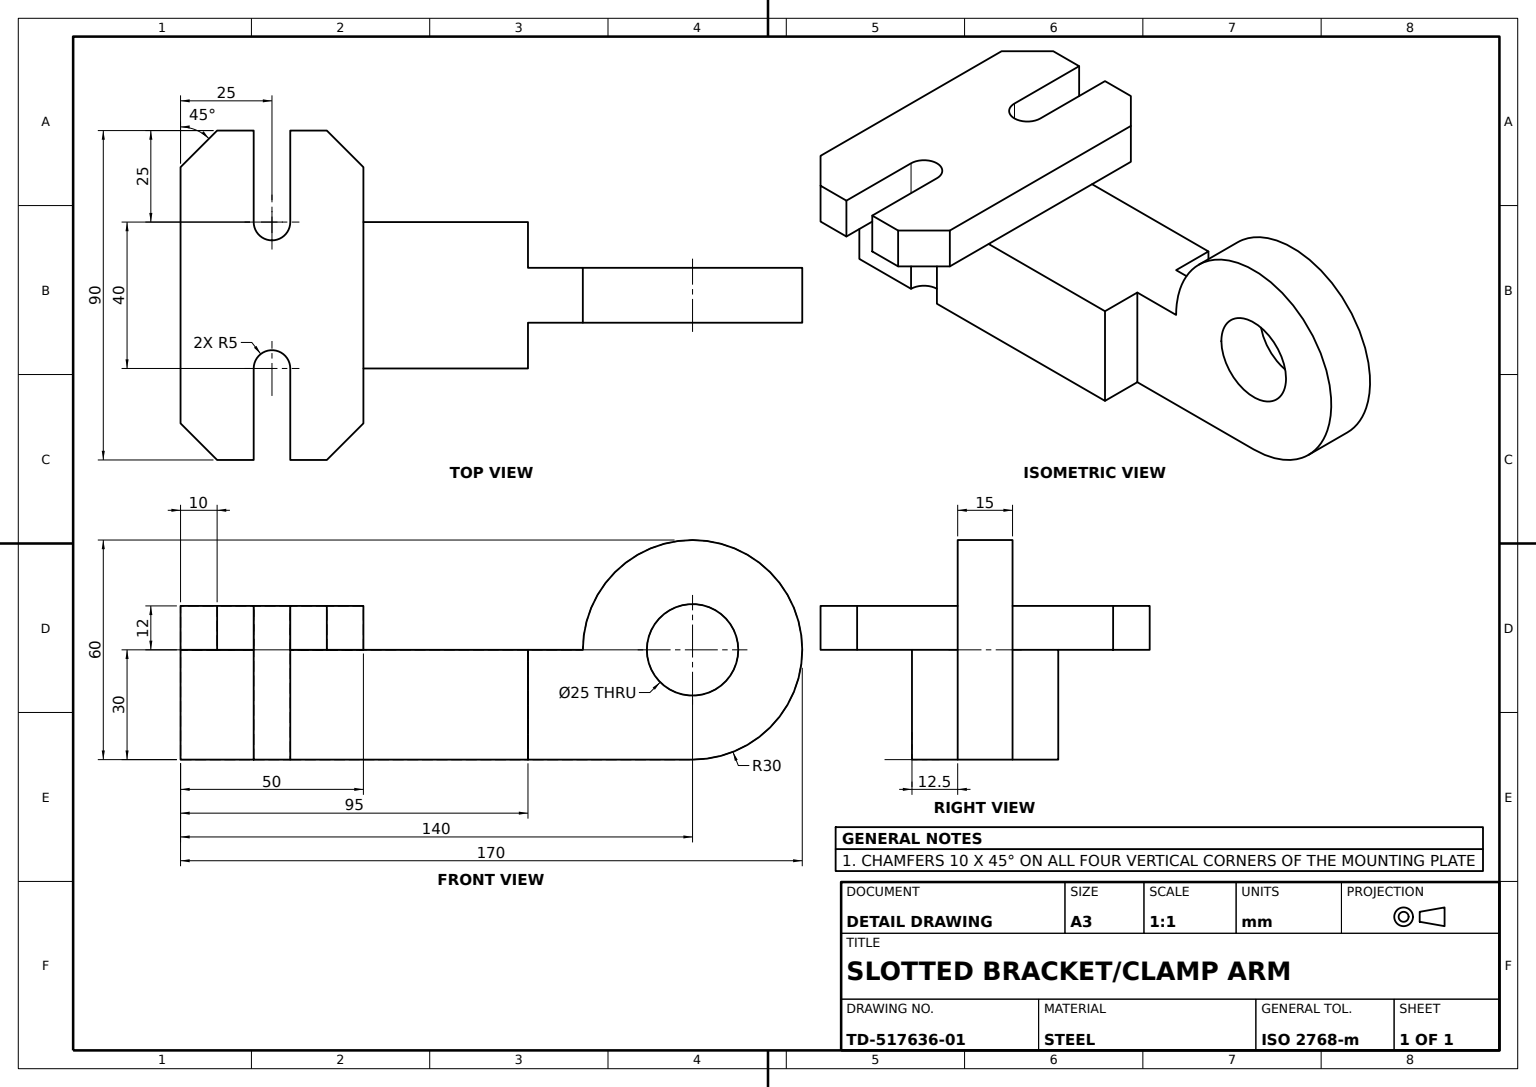
SolidWorks part; units mm, degrees
material "Plain Carbon Steel"
ref_plane "Front Plane" through (0, 0, 0) normal (0, 0, 1) x (1, 0, 0)
ref_plane "Top Plane" through (0, 0, 0) normal (0, 1, 0) x (1, 0, 0)
ref_plane "Right Plane" through (0, 0, 0) normal (1, 0, 0) x (0, 0, -1)
sketch "Rod Body Sketch" plane through (0, 0, 0) normal (0, 0, 1) x (1, 0, 0)
  line L1 (-47.5, -15) -> (47.5, -15)
  line L2 (-47.5, -15) -> (-47.5, 15)
  line L3 (-47.5, 15) -> (47.5, 15)
  line L4 (47.5, -15) -> (47.5, 15)
  line L5 (-47.5, -15) -> (47.5, 15) construction
  line L6 (-47.5, 15) -> (47.5, -15) construction
  point P0 (0, 0)
  dimension "D1" = 30
  dimension "D2" = 95
extrude "Rod Body 30x95" add sketch "Rod Body Sketch" along normal mid plane 40
sketch "Mounting Plate Sketch" plane through (0, 15, 0) normal (0, 1, 0) x (1, 0, 0)
  line L0 (0, 0) -> (-9.5797, 0) construction
  line L1 (-47.5, 45) -> (2.5, 45)
  line L2 (-47.5, 45) -> (-47.5, -45)
  line L3 (-47.5, -45) -> (2.5, -45)
  line L4 (2.5, 45) -> (2.5, -45)
  line L5 (47.5, -20) -> (47.5, 20) construction
  dimension "D1" = 90
  dimension "D2" = 50
  dimension "D3" = 45
extrude "Mounting Plate 12mm" add sketch "Mounting Plate Sketch" along normal blind 12
sketch "Eye Boss Sketch" plane through (0, 0, 0) normal (0, 0, 1) x (1, 0, 0)
  line L0 (-47.5, 15) -> (-47.5, -15) construction
  line L1 (92.5, -15) -> (47.5, -15)
  line L2 (47.5, -15) -> (47.5, 15)
  line L3 (47.5, 15) -> (62.5, 15)
  arc A0 (92.5, -15) -> (62.5, 15) centre (92.5, 15) ccw
  dimension "D1" = 60
  dimension "D2" = 140
extrude "Eye Boss" add sketch "Eye Boss Sketch" along normal mid plane 15
sketch "Eye Hole Sketch" plane through (0, 0, 7.5) normal (0, 0, 1) x (1, 0, 0)
  circle A0 centre (92.5, 15) radius 12.5
  dimension "D1" = 25
extrude "Eye Hole Ø25" cut sketch "Eye Hole Sketch" against normal blind 15
sketch "Mounting Slots Sketch" plane through (0, 27, 0) normal (0, 1, 0) x (1, 0, 0)
  line L0 (2.5, 45) -> (-47.5, 45) construction
  line L1 (-47.5, -45) -> (2.5, -45) construction
  line L2 (-27.5, 20) -> (-27.5, 45)
  line L3 (-27.5, 45) -> (-17.5, 45)
  line L4 (-17.5, 45) -> (-17.5, 20)
  line L5 (-27.5, -20) -> (-27.5, -45)
  line L6 (-27.5, -45) -> (-17.5, -45)
  line L7 (-17.5, -45) -> (-17.5, -20)
  arc A0 (-27.5, 20) -> (-17.5, 20) centre (-22.5, 20) ccw
  arc A1 (-17.5, -20) -> (-27.5, -20) centre (-22.5, -20) ccw
  point P8 (-22.5, 45)
  dimension "D1" = 10
  dimension "D2" = 25
  dimension "D3" = 25
extrude "Mounting Slots 2x10" cut sketch "Mounting Slots Sketch" against normal through all
chamfer "Plate Corner Chamfers 10x45" distance 10 angle 45 4 edges at (2.5, 21, -45) (-47.5, 21, -45) (2.5, 21, 45) (-47.5, 21, 45)
